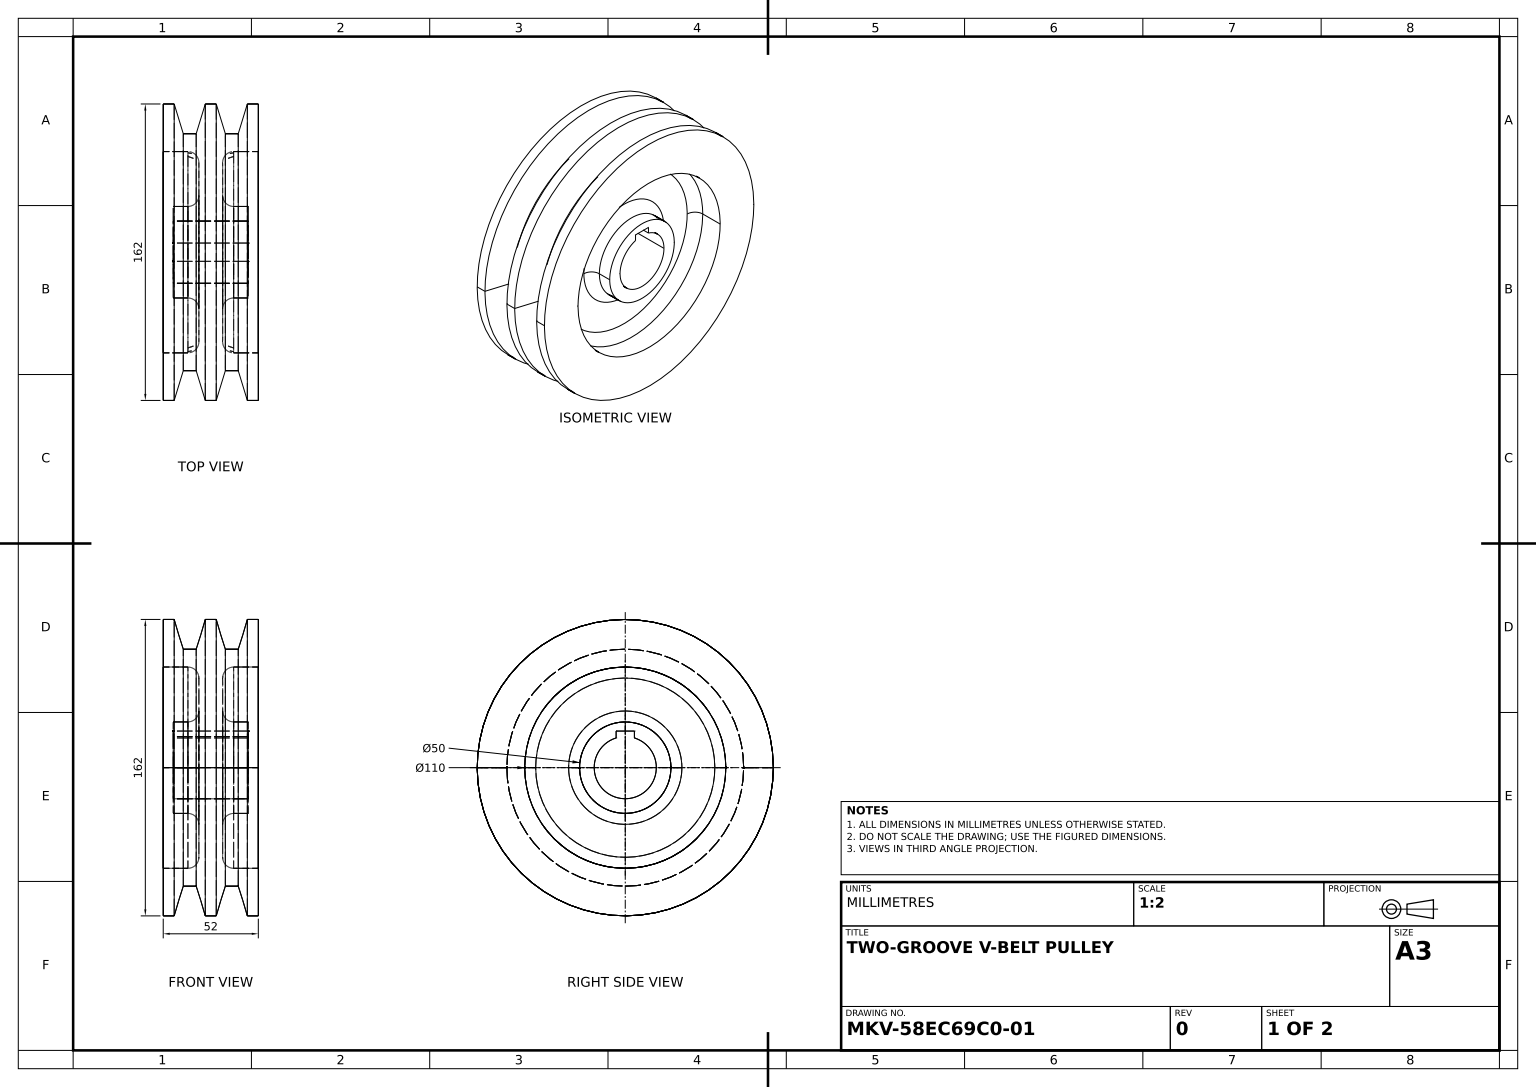
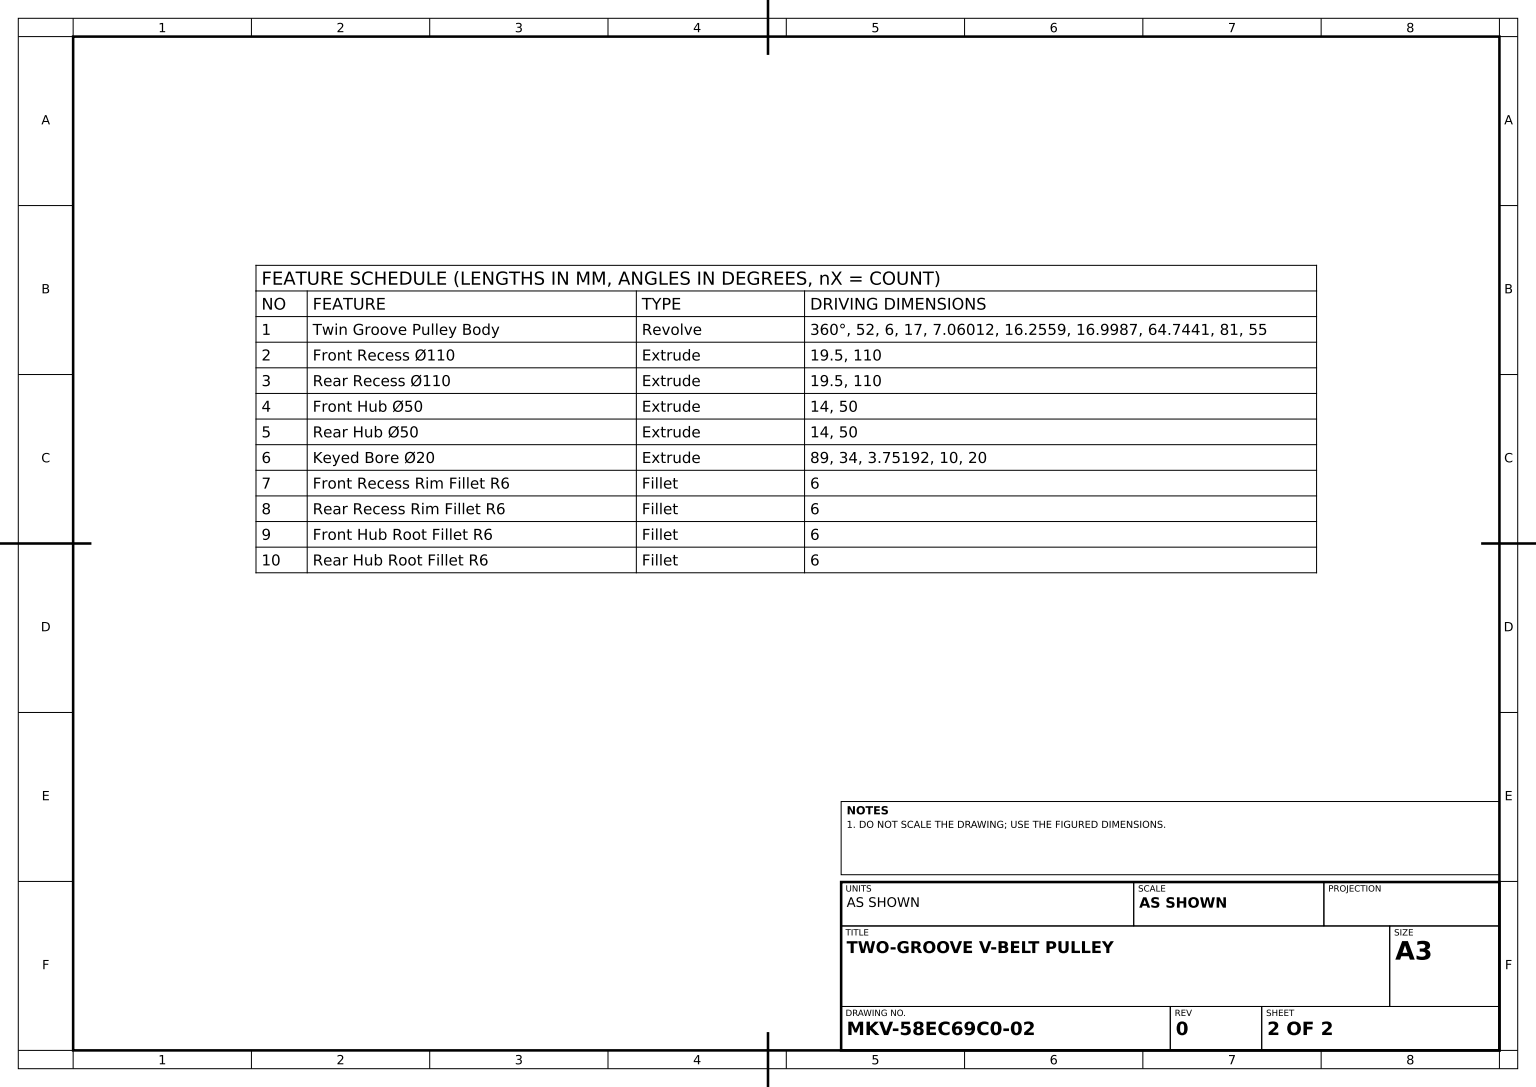
from build123d import *

# Parameters (mm, degrees)
FRONT_RECESS_110_SKETCH_R    = 55
FRONT_RECESS_110_DEPTH       = 19.5
REAR_START                   = -19.5
REAR_RECESS_110_SKETCH_R     = 55
REAR_RECESS_110_DEPTH        = 19.5
FRONT_HUB_50_SKETCH_R        = 25
FRONT_HUB_50_DEPTH           = 14
REAR_START_2                 = 14
REAR_HUB_50_SKETCH_R         = 25
REAR_HUB_50_DEPTH            = 14
KEYED_BORE_20_DEPTH          = 89
FRONT_RECESS_RIM_FILLET_R6_R = 6
REAR_RECESS_RIM_FILLET_R6_R  = 6
FRONT_HUB_ROOT_FILLET_R6_R   = 6
REAR_HUB_ROOT_FILLET_R6_R    = 6


with BuildPart() as part:
    # Pulley Rim Profile Sketch → Twin Groove Pulley Body (revolve)
    with BuildSketch(Plane.XY, mode=Mode.PRIVATE) as twin_groove_pulley_body_sk:
        Polygon((52, 0), (0, 0), (0, 81), (6, 81), (10.969940868, 64.744055898), (18.030059132, 64.744055898), (23, 81), (29, 81), (33.969940868, 64.744055898), (41.030059132, 64.744055898), (46, 81), (52, 81), align=None)
    revolve(twin_groove_pulley_body_sk.sketch.rotate(Axis((52, 0, 0), (-1, 0, 0)), 90), axis=Axis((52, 0, 0), (-1, 0, 0)))

    # Front Recess Ø110 Sketch → Front Recess Ø110 (cut)
    with BuildSketch(Plane(origin=(52, 0, 0), x_dir=(0, 0, -1), z_dir=(1, 0, 0))):
        Circle(FRONT_RECESS_110_SKETCH_R)
    extrude(amount=-FRONT_RECESS_110_DEPTH, mode=Mode.SUBTRACT)

    # Rear Recess Ø110 Sketch → Rear Recess Ø110 (cut)
    with BuildSketch(Plane.ZY.offset(REAR_START)):
        with Locations(Location((0, 0, 0), (0, 0, 180))):
            Circle(REAR_RECESS_110_SKETCH_R)
    extrude(amount=REAR_RECESS_110_DEPTH, mode=Mode.SUBTRACT)

    # Front Hub Ø50 Sketch → Front Hub Ø50 (add)
    with BuildSketch(Plane(origin=(32.5, 0, 0), x_dir=(0, 0, -1), z_dir=(1, 0, 0))):
        Circle(FRONT_HUB_50_SKETCH_R)
    extrude(amount=FRONT_HUB_50_DEPTH)

    # Rear Hub Ø50 Sketch → Rear Hub Ø50 (add)
    with BuildSketch(Plane.ZY.offset(-19.5).offset(REAR_START_2)):
        with Locations(Location((0, 0, 0), (0, 0, 180))):
            Circle(REAR_HUB_50_SKETCH_R)
    extrude(amount=-REAR_HUB_50_DEPTH)

    # Keyed Bore Ø20 Sketch → Keyed Bore Ø20 (cut)
    with BuildSketch(Plane.ZY.offset(-5.5)):
        with BuildLine():
            Line((0, 20), (5, 20))
            Line((5, 20), (5, 16.248076809))
            ThreePointArc((5, 16.248076809), (0, -17), (-5, 16.248076809))
            Line((-5, 16.248076809), (-5, 20))
            Line((-5, 20), (0, 20))
        make_face()
    extrude(amount=-KEYED_BORE_20_DEPTH, mode=Mode.SUBTRACT)

    # Front Recess Rim Fillet R6
    front_recess_rim_fillet_r6_edges = [part.edges().sort_by_distance(p)[0] for p in [
        (32.5, 0, 55),
    ]]
    fillet(front_recess_rim_fillet_r6_edges, radius=FRONT_RECESS_RIM_FILLET_R6_R)

    # Rear Recess Rim Fillet R6
    rear_recess_rim_fillet_r6_edges = [part.edges().sort_by_distance(p)[0] for p in [
        (19.5, 0, 55),
    ]]
    fillet(rear_recess_rim_fillet_r6_edges, radius=REAR_RECESS_RIM_FILLET_R6_R)

    # Front Hub Root Fillet R6
    front_hub_root_fillet_r6_edges = [part.edges().sort_by_distance(p)[0] for p in [
        (32.5, 0, 25),
    ]]
    fillet(front_hub_root_fillet_r6_edges, radius=FRONT_HUB_ROOT_FILLET_R6_R)

    # Rear Hub Root Fillet R6
    rear_hub_root_fillet_r6_edges = [part.edges().sort_by_distance(p)[0] for p in [
        (19.5, 0, 25),
    ]]
    fillet(rear_hub_root_fillet_r6_edges, radius=REAR_HUB_ROOT_FILLET_R6_R)


solid = part.part
